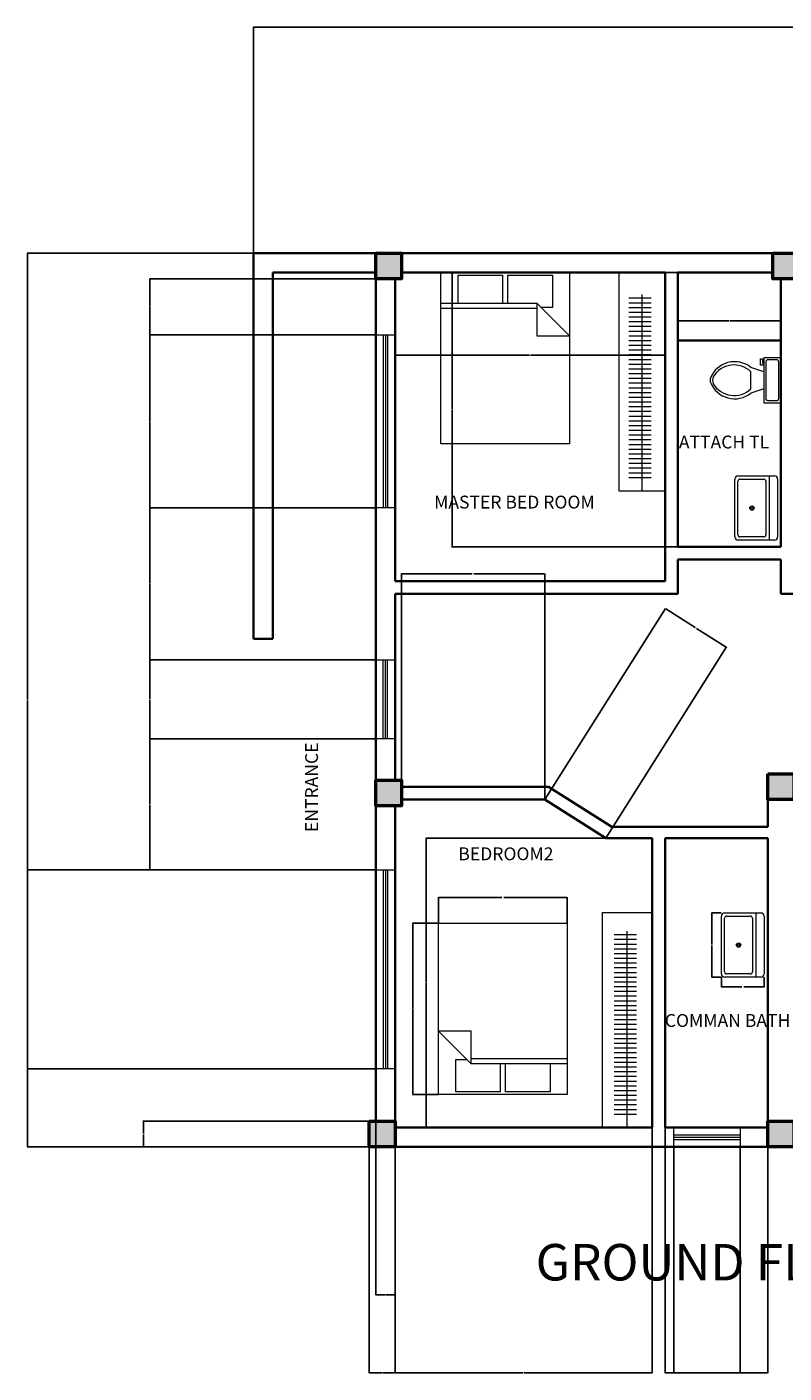
# Model space of a CAD drawing. Units: inches. Extents: x 369 to 4994, y 516 to 1297.
# Tile 1 of 9: x 369 to 722, y 516 to 1144. Entities that reach past the tile are written whole.
import ezdxf

# ---------------------------------------------------------------- set-up
doc = ezdxf.new("R2010")
doc.units = ezdxf.units.IN
doc.header["$MEASUREMENT"] = 0
for name, color, linetype, lineweight in [('A-ANNO-DIMS', 2, 'Continuous', 18), ('A-ANNO-TEXT', 7, 'Continuous', 35), ('A-AREA-IDEN', 7, 'Continuous', 18), ('A-COLS', 7, 'Continuous', 50), ('A-FLOR-CASE', 8, 'Continuous', 18), ('A-FLOR-CASE-PATT', 252, 'Continuous', 13), ('A-FLOR-FIXT', 9, 'Continuous', 18), ('A-FLOR-STRS', 3, 'Continuous', 25), ('A-FURN', 8, 'Continuous', 18), ('A-GLAZ', 4, 'Continuous', 18), ('A-WALL', 7, 'Continuous', 35)]:
    doc.layers.add(name, color=color, linetype=linetype, lineweight=lineweight)
doc.layers.add('A-COLS-PATT', color=18, linetype='Continuous', lineweight=13, true_color=0x000000)
doc.styles.get("Standard").update_dxf_attribs({"font": 'arial.ttf'})
doc.dimstyles.get("Standard").update_dxf_attribs({"dimtxt": 0.18, "dimasz": 0.18, "dimexe": 0.18, "dimexo": 0.0625, "dimgap": 0.09, "dimtad": 0, "dimtih": 1, "dimtoh": 1, "dimdec": 4, "dimzin": 0, "dimdsep": 46, "dimtxsty": 'Standard', "dimcen": 0.09, "dimadec": 0, "dimazin": 0, "dimtfac": 1, "dimtdec": 4, "dimtofl": 0, "dimtmove": 0, "dimatfit": 3, "dimfxl": 1, "dimtolj": 1, "dimtzin": 0, "dimarcsym": 0})

# ---------------------------------------------------------------- blocks, each defined once
blk = doc.blocks.new('Bed - Queen')
for p, q in [((0, -80.00003), (0, 0)), ((0, 0), (59.99999, 0)), ((59.99999, 0), (59.99999, -80.00003)), ((7.99999, -1.2), (28.79998, -1.2)), ((7.99999, -14.4), (7.99999, -1.2)), ((28.79998, -1.2), (28.79998, -14.4)), ((31.19999, -1.2), (51.99999, -1.2)), ((31.19999, -14.4), (31.19999, -1.2)), ((51.99999, -1.2), (51.99999, -16.4)), ((0, -14.4), (44.8, -14.4)), ((44.8, -16.8), (0, -16.8)), ((59.99999, -29.6), (44.8, -14.4)), ((44.8, -14.4), (44.8, -29.6)), ((51.99999, -16.4), (46.79936, -16.4)), ((44.8, -29.6), (59.99999, -29.6)), ((59.99999, -80.00003), (0, -80.00003))]:
    blk.add_line(p, q)
blk = doc.blocks.new('Toilet - top')
for p, q in [((9.5, -6), (9.5, -2)), ((-10, -8.5), (-8, -8.5)), ((-10, -9.5), (-10, -8.5)), ((-7, -9.5), (-10, -9.5)), ((-8, -8.5), (-8, -8)), ((-7, -8), (-7, -9.5)), ((-4, -8), (-6, -14)), ((4, -8), (6, -14)), ((4, -14), (-4, -14))]:
    blk.add_line(p, q)
blk.add_lwpolyline([(10.5, -8), (10.5, 0), (-10.5, 0), (-10.5, -8)], close=True)
for points in [[(-9.5, -2), (-9.5, -6)], [(8.5, -1), (-8.5, -1)], [(-8.5, -7), (8.5, -7)]]:
    blk.add_lwpolyline(points)
for centre, radius, start, end in [((-8.62, -1.88), 0.884, 81.8699, 188.1301), ((-8.62, -6.12), 0.884, 171.8699, 278.1301), ((8.62, -1.88), 0.884, 351.8699, 98.1301), ((8.62, -6.12), 0.884, 261.8699, 8.1301), ((3.52, -21.58), 12.17, 141.46911, 247.97143), ((4.2, -21.82), 11.33, 136.36773, 238.94682), ((-3.52, -21.58), 12.17, 292.02843, 38.53071), ((-4.2, -21.82), 11.33, 301.05301, 43.63209), ((0, -27.88), 4, 245.73182, 294.26817), ((0, -29), 4, 254.86053, 285.13947)]:
    blk.add_arc(centre, radius, start, end)
blk = doc.blocks.new('Sink-single - 30 in top')
blk.add_line((-15, -3.999996), (15, -3.999996))
for points in [[(-13.5, 0), (13.5, 0)], [(-15, -18.499996), (-15, -1.5)], [(-12.5, -5.499996), (12.5, -5.499996)], [(15, -1.5), (15, -18.499996)], [(-13.5, -17.499996), (-13.5, -6.499996)], [(13.5, -6.499996), (13.5, -17.499996)], [(12.5, -18.499996), (-12.5, -18.499996)], [(13.5, -19.999996), (-13.5, -19.999996)]]:
    blk.add_lwpolyline(points)
for radius in [1, 0.5]:
    blk.add_circle((0, -11.999996), radius)
for centre, radius, start, end in [((-13.5, -1.5), 1.5, 90, 180), ((-12.5, -6.499996), 1, 90, 180), ((12.5, -6.499996), 1, 0, 90), ((13.5, -1.5), 1.5, 0, 90), ((-13.5, -18.499996), 1.5, 180, 270), ((-12.5, -17.499996), 1, 180, 270), ((12.5, -17.499996), 1, 270, 0), ((13.5, -18.499996), 1.5, 270, 0)]:
    blk.add_arc(centre, radius, start, end)
blk = doc.blocks.new('BALCONY-EDGE')
for p, q in [((57, 180), (0, 180)), ((0, 180), (0, 0)), ((9, 171), (9, 0)), ((57, 171), (9, 171)), ((9, 0), (0, 0))]:
    blk.add_line(p, q)
blk = doc.blocks.new('*D19')
at = {"layer": 'A-ANNO-DIMS', "color": 0, "lineweight": -2, "transparency": 16777216}
for p, q in [((560.51, 726.18), (548.39, 726.18)), ((548.57, 726), (548.57, 686.37)), ((548.57, 646.36), (548.57, 685.99)), ((560.51, 646.18), (548.39, 646.18))]:
    blk.add_line(p, q, dxfattribs=at)
at = {"layer": 'A-ANNO-DIMS', "color": 0, "transparency": 16777216}
for points in [[(548.54, 726), (548.6, 726), (548.57, 726.18)], [(548.54, 646.36), (548.6, 646.36), (548.57, 646.18)]]:
    blk.add_solid(points, dxfattribs=at)
at = {"layer": 'Defpoints', "color": 0, "transparency": 16777216}
for p in [(560.57, 726.18), (548.57, 646.18), (560.57, 646.18)]:
    blk.add_point(p, dxfattribs=at)
at = {"layer": 'A-ANNO-DIMS', "color": 0, "transparency": 16777216, "insert": (548.57, 686.18), "char_height": 0.18, "attachment_point": 5}
blk.add_mtext('\\A1;QUEEN BED 80 TYP.', dxfattribs=at)
blk = doc.blocks.new('*D20')
at = {"layer": 'A-ANNO-DIMS', "color": 0, "lineweight": -2, "transparency": 16777216}
for p, q in [((560.57, 726.24), (560.57, 738.36)), ((560.75, 738.18), (590.05, 738.18)), ((620.39, 738.18), (591.1, 738.18)), ((620.57, 726.24), (620.57, 738.36))]:
    blk.add_line(p, q, dxfattribs=at)
at = {"layer": 'A-ANNO-DIMS', "color": 0, "transparency": 16777216}
for points in [[(560.75, 738.21), (560.75, 738.15), (560.57, 738.18)], [(620.39, 738.21), (620.39, 738.15), (620.57, 738.18)]]:
    blk.add_solid(points, dxfattribs=at)
at = {"layer": 'Defpoints', "color": 0, "transparency": 16777216}
for p in [(560.57, 738.18), (560.57, 726.18), (620.57, 726.18)]:
    blk.add_point(p, dxfattribs=at)
at = {"layer": 'A-ANNO-DIMS', "color": 0, "transparency": 16777216, "insert": (590.57, 738.18), "char_height": 0.18, "attachment_point": 5}
blk.add_mtext('\\A1;60 TYP.', dxfattribs=at)
blk = doc.blocks.new('*D27')
at = {"layer": 'A-ANNO-DIMS', "color": 0, "lineweight": -2, "transparency": 16777216}
for p, q in [((692.45, 730.94), (687.83, 730.94)), ((688.01, 730.76), (688.01, 716.12)), ((688.01, 701.12), (688.01, 715.75)), ((692.45, 700.94), (687.83, 700.94))]:
    blk.add_line(p, q, dxfattribs=at)
at = {"layer": 'A-ANNO-DIMS', "color": 0, "transparency": 16777216}
for points in [[(687.98, 730.76), (688.04, 730.76), (688.01, 730.94)], [(687.98, 701.12), (688.04, 701.12), (688.01, 700.94)]]:
    blk.add_solid(points, dxfattribs=at)
at = {"layer": 'Defpoints', "color": 0, "transparency": 16777216}
for p in [(692.51, 730.94), (688.01, 700.94), (692.51, 700.94)]:
    blk.add_point(p, dxfattribs=at)
at = {"layer": 'A-ANNO-DIMS', "color": 0, "transparency": 16777216, "insert": (688.01, 715.94), "char_height": 0.18, "attachment_point": 5}
blk.add_mtext('\\A1;SINK 30 TYP.', dxfattribs=at)
blk = doc.blocks.new('*D28')
at = {"layer": 'A-ANNO-DIMS', "color": 0, "lineweight": -2, "transparency": 16777216}
for p, q in [((692.51, 700.88), (692.51, 696.26)), ((712.51, 700.88), (712.51, 696.26)), ((692.69, 696.44), (701.98, 696.44)), ((712.33, 696.44), (703.04, 696.44))]:
    blk.add_line(p, q, dxfattribs=at)
at = {"layer": 'A-ANNO-DIMS', "color": 0, "transparency": 16777216}
for points in [[(692.69, 696.47), (692.69, 696.41), (692.51, 696.44)], [(712.33, 696.47), (712.33, 696.41), (712.51, 696.44)]]:
    blk.add_solid(points, dxfattribs=at)
at = {"layer": 'Defpoints', "color": 0, "transparency": 16777216}
for p in [(692.51, 700.94), (712.51, 700.94), (712.51, 696.44)]:
    blk.add_point(p, dxfattribs=at)
at = {"layer": 'A-ANNO-DIMS', "color": 0, "transparency": 16777216, "insert": (702.51, 696.44), "char_height": 0.18, "attachment_point": 5}
blk.add_mtext('\\A1;20 TYP.', dxfattribs=at)
blk = doc.blocks.new('*D39')
at = {"layer": 'A-ANNO-DIMS', "color": 0, "lineweight": -2, "transparency": 16777216}
for p, q in [((474.26, 1038.85), (474.26, 1144.37)), ((474.44, 1144.19), (760.47, 1144.19)), ((1047.08, 1144.19), (761.05, 1144.19)), ((1047.26, 1038.85), (1047.26, 1144.37))]:
    blk.add_line(p, q, dxfattribs=at)
at = {"layer": 'A-ANNO-DIMS', "color": 0, "transparency": 16777216}
for points in [[(474.44, 1144.22), (474.44, 1144.16), (474.26, 1144.19)], [(1047.08, 1144.22), (1047.08, 1144.16), (1047.26, 1144.19)]]:
    blk.add_solid(points, dxfattribs=at)
at = {"layer": 'Defpoints', "color": 0, "transparency": 16777216}
for p in [(1047.26, 1144.19), (474.26, 1038.79), (1047.26, 1038.79)]:
    blk.add_point(p, dxfattribs=at)
at = {"layer": 'A-ANNO-DIMS', "color": 0, "transparency": 16777216, "insert": (760.76, 1144.19), "char_height": 0.18, "attachment_point": 5}
blk.add_mtext('\\A1;573', dxfattribs=at)
blk = doc.blocks.new('*D40')
at = {"layer": 'A-ANNO-DIMS', "color": 0, "lineweight": -2, "transparency": 16777216}
for p, q in [((474.2, 1038.79), (368.68, 1038.79)), ((368.86, 1038.61), (368.86, 830.47)), ((368.86, 621.97), (368.86, 830.11)), ((528.2, 621.79), (368.68, 621.79))]:
    blk.add_line(p, q, dxfattribs=at)
at = {"layer": 'A-ANNO-DIMS', "color": 0, "transparency": 16777216}
for points in [[(368.83, 1038.61), (368.89, 1038.61), (368.86, 1038.79)], [(368.83, 621.97), (368.89, 621.97), (368.86, 621.79)]]:
    blk.add_solid(points, dxfattribs=at)
at = {"layer": 'Defpoints', "color": 0, "transparency": 16777216}
for p in [(368.86, 1038.79), (474.26, 1038.79), (528.26, 621.79)]:
    blk.add_point(p, dxfattribs=at)
at = {"layer": 'A-ANNO-DIMS', "color": 0, "transparency": 16777216, "insert": (368.86, 830.29), "char_height": 0.18, "attachment_point": 5}
blk.add_mtext('\\A1;417', dxfattribs=at)
blk = doc.blocks.new('*D41')
at = {"layer": 'A-ANNO-DIMS', "color": 0, "lineweight": -2, "transparency": 16777216}
for p, q in [((540.26, 885.85), (540.26, 991.37)), ((540.44, 991.19), (602.98, 991.19)), ((666.08, 991.19), (603.54, 991.19)), ((666.26, 885.85), (666.26, 991.37))]:
    blk.add_line(p, q, dxfattribs=at)
at = {"layer": 'A-ANNO-DIMS', "color": 0, "transparency": 16777216}
for points in [[(540.44, 991.22), (540.44, 991.16), (540.26, 991.19)], [(666.08, 991.22), (666.08, 991.16), (666.26, 991.19)]]:
    blk.add_solid(points, dxfattribs=at)
at = {"layer": 'Defpoints', "color": 0, "transparency": 16777216}
for p in [(666.26, 991.19), (540.26, 885.79), (666.26, 885.79)]:
    blk.add_point(p, dxfattribs=at)
at = {"layer": 'A-ANNO-DIMS', "color": 0, "transparency": 16777216, "insert": (603.26, 991.19), "char_height": 0.18, "attachment_point": 5}
blk.add_mtext('\\A1;126', dxfattribs=at)
blk = doc.blocks.new('*D42')
at = {"layer": 'A-ANNO-DIMS', "color": 0, "lineweight": -2, "transparency": 16777216}
for p, q in [((672.26, 901.88), (672.26, 1007.4)), ((672.44, 1007.22), (696.04, 1007.22)), ((720.08, 1007.22), (696.48, 1007.22)), ((720.26, 901.88), (720.26, 1007.4))]:
    blk.add_line(p, q, dxfattribs=at)
at = {"layer": 'A-ANNO-DIMS', "color": 0, "transparency": 16777216}
for points in [[(672.44, 1007.25), (672.44, 1007.19), (672.26, 1007.22)], [(720.08, 1007.25), (720.08, 1007.19), (720.26, 1007.22)]]:
    blk.add_solid(points, dxfattribs=at)
at = {"layer": 'Defpoints', "color": 0, "transparency": 16777216}
for p in [(720.26, 1007.22), (672.26, 901.82), (720.26, 901.82)]:
    blk.add_point(p, dxfattribs=at)
at = {"layer": 'A-ANNO-DIMS', "color": 0, "transparency": 16777216, "insert": (696.26, 1007.22), "char_height": 0.18, "attachment_point": 5}
blk.add_mtext('\\A1;48', dxfattribs=at)
blk = doc.blocks.new('*D48')
at = {"layer": 'A-ANNO-DIMS', "color": 0, "lineweight": -2, "transparency": 16777216}
for p, q in [((540.26, 630.73), (540.26, 516.21)), ((660.26, 630.73), (660.26, 516.21)), ((540.44, 516.39), (599.98, 516.39)), ((660.08, 516.39), (600.54, 516.39))]:
    blk.add_line(p, q, dxfattribs=at)
at = {"layer": 'A-ANNO-DIMS', "color": 0, "transparency": 16777216}
for points in [[(540.44, 516.42), (540.44, 516.36), (540.26, 516.39)], [(660.08, 516.42), (660.08, 516.36), (660.26, 516.39)]]:
    blk.add_solid(points, dxfattribs=at)
at = {"layer": 'Defpoints', "color": 0, "transparency": 16777216}
for p in [(540.26, 630.79), (660.26, 630.79), (660.26, 516.39)]:
    blk.add_point(p, dxfattribs=at)
at = {"layer": 'A-ANNO-DIMS', "color": 0, "transparency": 16777216, "insert": (600.26, 516.39), "char_height": 0.18, "attachment_point": 5}
blk.add_mtext('\\A1;120', dxfattribs=at)
blk = doc.blocks.new('*D49')
at = {"layer": 'A-ANNO-DIMS', "color": 0, "lineweight": -2, "transparency": 16777216}
for p, q in [((666.26, 630.73), (666.26, 516.21)), ((714.26, 630.73), (714.26, 516.21)), ((666.44, 516.39), (690.04, 516.39)), ((714.08, 516.39), (690.48, 516.39))]:
    blk.add_line(p, q, dxfattribs=at)
at = {"layer": 'A-ANNO-DIMS', "color": 0, "transparency": 16777216}
for points in [[(666.44, 516.42), (666.44, 516.36), (666.26, 516.39)], [(714.08, 516.42), (714.08, 516.36), (714.26, 516.39)]]:
    blk.add_solid(points, dxfattribs=at)
at = {"layer": 'Defpoints', "color": 0, "transparency": 16777216}
for p in [(666.26, 630.79), (714.26, 630.79), (714.26, 516.39)]:
    blk.add_point(p, dxfattribs=at)
at = {"layer": 'A-ANNO-DIMS', "color": 0, "transparency": 16777216, "insert": (690.26, 516.39), "char_height": 0.18, "attachment_point": 5}
blk.add_mtext('\\A1;48', dxfattribs=at)
blk = doc.blocks.new('*D53')
at = {"layer": 'A-ANNO-DIMS', "color": 0, "lineweight": -2, "transparency": 16777216}
for p, q in [((672.2, 1029.79), (566.68, 1029.79)), ((566.86, 1029.61), (566.86, 965.99)), ((566.86, 902), (566.86, 965.62)), ((672.2, 901.82), (566.68, 901.82))]:
    blk.add_line(p, q, dxfattribs=at)
at = {"layer": 'A-ANNO-DIMS', "color": 0, "transparency": 16777216}
for points in [[(566.83, 1029.61), (566.89, 1029.61), (566.86, 1029.79)], [(566.83, 902), (566.89, 902), (566.86, 901.82)]]:
    blk.add_solid(points, dxfattribs=at)
at = {"layer": 'Defpoints', "color": 0, "transparency": 16777216}
for p in [(566.86, 1029.79), (672.26, 1029.79), (672.26, 901.82)]:
    blk.add_point(p, dxfattribs=at)
at = {"layer": 'A-ANNO-DIMS', "color": 0, "transparency": 16777216, "insert": (566.86, 965.8), "char_height": 0.18, "attachment_point": 5}
blk.add_mtext('\\A1;127.97', dxfattribs=at)
blk = doc.blocks.new('*D56')
at = {"layer": 'A-ANNO-DIMS', "color": 0, "lineweight": -2, "transparency": 16777216}
for p, q in [((660.2, 765.79), (554.68, 765.79)), ((554.86, 765.61), (554.86, 698.47)), ((554.86, 630.97), (554.86, 698.11)), ((660.2, 630.79), (554.68, 630.79))]:
    blk.add_line(p, q, dxfattribs=at)
at = {"layer": 'A-ANNO-DIMS', "color": 0, "transparency": 16777216}
for points in [[(554.83, 765.61), (554.89, 765.61), (554.86, 765.79)], [(554.83, 630.97), (554.89, 630.97), (554.86, 630.79)]]:
    blk.add_solid(points, dxfattribs=at)
at = {"layer": 'Defpoints', "color": 0, "transparency": 16777216}
for p in [(554.86, 765.79), (660.26, 765.79), (660.26, 630.79)]:
    blk.add_point(p, dxfattribs=at)
at = {"layer": 'A-ANNO-DIMS', "color": 0, "transparency": 16777216, "insert": (554.86, 698.29), "char_height": 0.18, "attachment_point": 5}
blk.add_mtext('\\A1;135', dxfattribs=at)
blk = doc.blocks.new('*D57')
at = {"layer": 'A-ANNO-DIMS', "color": 0, "lineweight": -2, "transparency": 16777216}
for p, q in [((543.26, 783.85), (543.26, 889.37)), ((543.44, 889.19), (576.28, 889.19)), ((609.9, 889.19), (577.07, 889.19)), ((610.08, 783.85), (610.08, 889.37))]:
    blk.add_line(p, q, dxfattribs=at)
at = {"layer": 'A-ANNO-DIMS', "color": 0, "transparency": 16777216}
for points in [[(543.44, 889.22), (543.44, 889.16), (543.26, 889.19)], [(609.9, 889.22), (609.9, 889.16), (610.08, 889.19)]]:
    blk.add_solid(points, dxfattribs=at)
at = {"layer": 'Defpoints', "color": 0, "transparency": 16777216}
for p in [(610.08, 889.19), (543.26, 783.79), (610.08, 783.79)]:
    blk.add_point(p, dxfattribs=at)
at = {"layer": 'A-ANNO-DIMS', "color": 0, "transparency": 16777216, "insert": (576.67, 889.19), "char_height": 0.18, "attachment_point": 5}
blk.add_mtext('\\A1;66.83', dxfattribs=at)
blk = doc.blocks.new('*D58')
at = {"layer": 'A-ANNO-DIMS', "color": 0, "lineweight": -2, "transparency": 16777216}
for p, q in [((610.12, 783.84), (666.48, 873.04)), ((666.54, 872.8), (680.34, 864.07)), ((694.72, 854.99), (680.92, 863.71)), ((638.61, 765.84), (694.97, 855.04))]:
    blk.add_line(p, q, dxfattribs=at)
at = {"layer": 'A-ANNO-DIMS', "color": 0, "transparency": 16777216}
for points in [[(666.55, 872.82), (666.52, 872.77), (666.39, 872.89)], [(694.74, 855.01), (694.7, 854.96), (694.87, 854.89)]]:
    blk.add_solid(points, dxfattribs=at)
at = {"layer": 'Defpoints', "color": 0, "transparency": 16777216}
for p in [(694.87, 854.89), (610.08, 783.79), (638.57, 765.79)]:
    blk.add_point(p, dxfattribs=at)
at = {"layer": 'A-ANNO-DIMS', "color": 0, "transparency": 16777216, "insert": (680.63, 863.89), "char_height": 0.18, "attachment_point": 5}
blk.add_mtext('\\A1;33.7', dxfattribs=at)
blk = doc.blocks.new('*D59')
at = {"layer": 'A-ANNO-DIMS', "color": 0, "lineweight": -2, "transparency": 16777216}
for p, q in [((531.2, 1026.79), (425.68, 1026.79)), ((425.86, 1026.61), (425.86, 1013.94)), ((425.86, 1000.91), (425.86, 1013.58)), ((531.2, 1000.73), (425.68, 1000.73))]:
    blk.add_line(p, q, dxfattribs=at)
at = {"layer": 'A-ANNO-DIMS', "color": 0, "transparency": 16777216}
for points in [[(425.83, 1026.61), (425.89, 1026.61), (425.86, 1026.79)], [(425.83, 1000.91), (425.89, 1000.91), (425.86, 1000.73)]]:
    blk.add_solid(points, dxfattribs=at)
at = {"layer": 'Defpoints', "color": 0, "transparency": 16777216}
for p in [(425.86, 1026.79), (531.26, 1026.79), (531.26, 1000.73)]:
    blk.add_point(p, dxfattribs=at)
at = {"layer": 'A-ANNO-DIMS', "color": 0, "transparency": 16777216, "insert": (425.86, 1013.76), "char_height": 0.18, "attachment_point": 5}
blk.add_mtext('\\A1;26.06', dxfattribs=at)
blk = doc.blocks.new('*D60')
at = {"layer": 'A-ANNO-DIMS', "color": 0, "lineweight": -2, "transparency": 16777216}
for p, q in [((531.2, 1000.73), (425.68, 1000.73)), ((425.86, 1000.55), (425.86, 960.54)), ((425.86, 920.17), (425.86, 960.18)), ((531.2, 919.99), (425.68, 919.99))]:
    blk.add_line(p, q, dxfattribs=at)
at = {"layer": 'A-ANNO-DIMS', "color": 0, "transparency": 16777216}
for points in [[(425.83, 1000.55), (425.89, 1000.55), (425.86, 1000.73)], [(425.83, 920.17), (425.89, 920.17), (425.86, 919.99)]]:
    blk.add_solid(points, dxfattribs=at)
at = {"layer": 'Defpoints', "color": 0, "transparency": 16777216}
for p in [(425.86, 1000.73), (531.26, 1000.73), (531.26, 919.99)]:
    blk.add_point(p, dxfattribs=at)
at = {"layer": 'A-ANNO-DIMS', "color": 0, "transparency": 16777216, "insert": (425.86, 960.36), "char_height": 0.18, "attachment_point": 5}
blk.add_mtext('\\A1;80.74', dxfattribs=at)
blk = doc.blocks.new('*D61')
at = {"layer": 'A-ANNO-DIMS', "color": 0, "lineweight": -2, "transparency": 16777216}
for p, q in [((531.2, 919.99), (425.68, 919.99)), ((425.86, 919.81), (425.86, 884.72)), ((425.86, 849.26), (425.86, 884.35)), ((531.2, 849.08), (425.68, 849.08))]:
    blk.add_line(p, q, dxfattribs=at)
at = {"layer": 'A-ANNO-DIMS', "color": 0, "transparency": 16777216}
for points in [[(425.83, 919.81), (425.89, 919.81), (425.86, 919.99)], [(425.83, 849.26), (425.89, 849.26), (425.86, 849.08)]]:
    blk.add_solid(points, dxfattribs=at)
at = {"layer": 'Defpoints', "color": 0, "transparency": 16777216}
for p in [(425.86, 919.99), (531.26, 919.99), (531.26, 849.08)]:
    blk.add_point(p, dxfattribs=at)
at = {"layer": 'A-ANNO-DIMS', "color": 0, "transparency": 16777216, "insert": (425.86, 884.54), "char_height": 0.18, "attachment_point": 5}
blk.add_mtext('\\A1;70.91', dxfattribs=at)
blk = doc.blocks.new('*D62')
at = {"layer": 'A-ANNO-DIMS', "color": 0, "lineweight": -2, "transparency": 16777216}
for p, q in [((531.2, 849.08), (425.68, 849.08)), ((425.86, 848.9), (425.86, 830.78)), ((425.86, 812.3), (425.86, 830.42)), ((531.2, 812.12), (425.68, 812.12))]:
    blk.add_line(p, q, dxfattribs=at)
at = {"layer": 'A-ANNO-DIMS', "color": 0, "transparency": 16777216}
for points in [[(425.83, 848.9), (425.89, 848.9), (425.86, 849.08)], [(425.83, 812.3), (425.89, 812.3), (425.86, 812.12)]]:
    blk.add_solid(points, dxfattribs=at)
at = {"layer": 'Defpoints', "color": 0, "transparency": 16777216}
for p in [(425.86, 849.08), (531.26, 849.08), (531.26, 812.12)]:
    blk.add_point(p, dxfattribs=at)
at = {"layer": 'A-ANNO-DIMS', "color": 0, "transparency": 16777216, "insert": (425.86, 830.6), "char_height": 0.18, "attachment_point": 5}
blk.add_mtext('\\A1;36.96', dxfattribs=at)
blk = doc.blocks.new('*D63')
at = {"layer": 'A-ANNO-DIMS', "color": 0, "lineweight": -2, "transparency": 16777216}
for p, q in [((531.2, 812.12), (425.68, 812.12)), ((425.86, 811.94), (425.86, 781.79)), ((425.86, 751.28), (425.86, 781.43)), ((531.2, 751.1), (425.68, 751.1))]:
    blk.add_line(p, q, dxfattribs=at)
at = {"layer": 'A-ANNO-DIMS', "color": 0, "transparency": 16777216}
for points in [[(425.83, 811.94), (425.89, 811.94), (425.86, 812.12)], [(425.83, 751.28), (425.89, 751.28), (425.86, 751.1)]]:
    blk.add_solid(points, dxfattribs=at)
at = {"layer": 'Defpoints', "color": 0, "transparency": 16777216}
for p in [(425.86, 812.12), (531.26, 812.12), (531.26, 751.1)]:
    blk.add_point(p, dxfattribs=at)
at = {"layer": 'A-ANNO-DIMS', "color": 0, "transparency": 16777216, "insert": (425.86, 781.61), "char_height": 0.18, "attachment_point": 5}
blk.add_mtext('\\A1;61.02', dxfattribs=at)
blk = doc.blocks.new('*D64')
at = {"layer": 'A-ANNO-DIMS', "color": 0, "lineweight": -2, "transparency": 16777216}
for p, q in [((531.2, 751.1), (368.68, 751.1)), ((368.86, 750.92), (368.86, 704.82)), ((368.86, 658.37), (368.86, 704.46)), ((531.2, 658.19), (368.68, 658.19))]:
    blk.add_line(p, q, dxfattribs=at)
at = {"layer": 'A-ANNO-DIMS', "color": 0, "transparency": 16777216}
for points in [[(368.83, 750.92), (368.89, 750.92), (368.86, 751.1)], [(368.83, 658.37), (368.89, 658.37), (368.86, 658.19)]]:
    blk.add_solid(points, dxfattribs=at)
at = {"layer": 'Defpoints', "color": 0, "transparency": 16777216}
for p in [(368.86, 751.1), (531.26, 751.1), (531.26, 658.19)]:
    blk.add_point(p, dxfattribs=at)
at = {"layer": 'A-ANNO-DIMS', "color": 0, "transparency": 16777216, "insert": (368.86, 704.64), "char_height": 0.18, "attachment_point": 5}
blk.add_mtext('\\A1;92.91', dxfattribs=at)
blk = doc.blocks.new('*D68')
at = {"layer": 'A-ANNO-DIMS', "color": 0, "lineweight": -2, "transparency": 16777216}
for p, q in [((670.31, 621.73), (670.31, 516.21)), ((701.35, 621.73), (701.35, 516.21)), ((670.49, 516.39), (685.44, 516.39)), ((701.17, 516.39), (686.22, 516.39))]:
    blk.add_line(p, q, dxfattribs=at)
at = {"layer": 'A-ANNO-DIMS', "color": 0, "transparency": 16777216}
for points in [[(670.49, 516.42), (670.49, 516.36), (670.31, 516.39)], [(701.17, 516.42), (701.17, 516.36), (701.35, 516.39)]]:
    blk.add_solid(points, dxfattribs=at)
at = {"layer": 'Defpoints', "color": 0, "transparency": 16777216}
for p in [(670.31, 621.79), (701.35, 621.79), (701.35, 516.39)]:
    blk.add_point(p, dxfattribs=at)
at = {"layer": 'A-ANNO-DIMS', "color": 0, "transparency": 16777216, "insert": (685.83, 516.39), "char_height": 0.18, "attachment_point": 5}
blk.add_mtext('\\A1;31.04', dxfattribs=at)
blk = doc.blocks.new('*D69')
at = {"layer": 'A-ANNO-DIMS', "color": 0, "lineweight": -2, "transparency": 16777216}
for p, q in [((528.26, 621.73), (528.26, 516.21)), ((540.26, 621.73), (540.26, 516.21)), ((528.44, 516.39), (534.05, 516.39)), ((540.08, 516.39), (534.47, 516.39))]:
    blk.add_line(p, q, dxfattribs=at)
at = {"layer": 'A-ANNO-DIMS', "color": 0, "transparency": 16777216}
for points in [[(528.44, 516.42), (528.44, 516.36), (528.26, 516.39)], [(540.08, 516.42), (540.08, 516.36), (540.26, 516.39)]]:
    blk.add_solid(points, dxfattribs=at)
at = {"layer": 'Defpoints', "color": 0, "transparency": 16777216}
for p in [(528.26, 621.79), (540.26, 621.79), (528.26, 516.39)]:
    blk.add_point(p, dxfattribs=at)
at = {"layer": 'A-ANNO-DIMS', "color": 0, "transparency": 16777216, "insert": (534.26, 516.39), "char_height": 0.18, "attachment_point": 5}
blk.add_mtext('\\A1;12', dxfattribs=at)
blk = doc.blocks.new('*D70')
at = {"layer": 'A-ANNO-DIMS', "color": 0, "lineweight": -2, "transparency": 16777216}
for p, q in [((528.2, 633.79), (422.68, 633.79)), ((422.86, 633.61), (422.86, 627.97)), ((422.86, 621.97), (422.86, 627.61)), ((528.2, 621.79), (422.68, 621.79))]:
    blk.add_line(p, q, dxfattribs=at)
at = {"layer": 'A-ANNO-DIMS', "color": 0, "transparency": 16777216}
for points in [[(422.83, 633.61), (422.89, 633.61), (422.86, 633.79)], [(422.83, 621.97), (422.89, 621.97), (422.86, 621.79)]]:
    blk.add_solid(points, dxfattribs=at)
at = {"layer": 'Defpoints', "color": 0, "transparency": 16777216}
for p in [(422.86, 633.79), (528.26, 633.79), (528.26, 621.79)]:
    blk.add_point(p, dxfattribs=at)
at = {"layer": 'A-ANNO-DIMS', "color": 0, "transparency": 16777216, "insert": (422.86, 627.79), "char_height": 0.18, "attachment_point": 5}
blk.add_mtext('\\A1;12', dxfattribs=at)
blk = doc.blocks.new('*D71')
at = {"layer": 'A-ANNO-DIMS', "color": 0, "lineweight": -2, "transparency": 16777216}
for p, q in [((531.26, 658.12), (531.26, 552.61)), ((540.26, 658.12), (540.26, 552.61)), ((531.44, 552.79), (535.61, 552.79)), ((540.08, 552.79), (535.91, 552.79))]:
    blk.add_line(p, q, dxfattribs=at)
at = {"layer": 'A-ANNO-DIMS', "color": 0, "transparency": 16777216}
for points in [[(531.44, 552.82), (531.44, 552.76), (531.26, 552.79)], [(540.08, 552.82), (540.08, 552.76), (540.26, 552.79)]]:
    blk.add_solid(points, dxfattribs=at)
at = {"layer": 'Defpoints', "color": 0, "transparency": 16777216}
for p in [(531.26, 658.19), (540.26, 658.19), (531.26, 552.79)]:
    blk.add_point(p, dxfattribs=at)
at = {"layer": 'A-ANNO-DIMS', "color": 0, "transparency": 16777216, "insert": (535.76, 552.79), "char_height": 0.18, "attachment_point": 5}
blk.add_mtext('\\A1;9', dxfattribs=at)
blk = doc.blocks.new('*D75')
at = {"layer": 'A-ANNO-DIMS', "color": 0, "lineweight": -2, "transparency": 16777216}
for p, q in [((1208.31, 1038.79), (368.68, 1038.79)), ((368.86, 1038.61), (368.86, 830.47)), ((368.86, 621.97), (368.86, 830.11)), ((1262.31, 621.79), (368.68, 621.79))]:
    blk.add_line(p, q, dxfattribs=at)
at = {"layer": 'A-ANNO-DIMS', "color": 0, "transparency": 16777216}
for points in [[(368.83, 1038.61), (368.89, 1038.61), (368.86, 1038.79)], [(368.83, 621.97), (368.89, 621.97), (368.86, 621.79)]]:
    blk.add_solid(points, dxfattribs=at)
at = {"layer": 'Defpoints', "color": 0, "transparency": 16777216}
for p in [(368.86, 1038.79), (1208.37, 1038.79), (1262.37, 621.79)]:
    blk.add_point(p, dxfattribs=at)
at = {"layer": 'A-ANNO-DIMS', "color": 0, "transparency": 16777216, "insert": (368.86, 830.29), "char_height": 0.18, "attachment_point": 5}
blk.add_mtext('\\A1;417', dxfattribs=at)
blk = doc.blocks.new('*D98')
at = {"layer": 'A-ANNO-DIMS', "color": 0, "lineweight": -2, "transparency": 16777216}
for p, q in [((1992.86, 1038.79), (368.68, 1038.79)), ((368.86, 1038.61), (368.86, 830.47)), ((368.86, 621.97), (368.86, 830.11)), ((2046.86, 621.79), (368.68, 621.79))]:
    blk.add_line(p, q, dxfattribs=at)
at = {"layer": 'A-ANNO-DIMS', "color": 0, "transparency": 16777216}
for points in [[(368.83, 1038.61), (368.89, 1038.61), (368.86, 1038.79)], [(368.83, 621.97), (368.89, 621.97), (368.86, 621.79)]]:
    blk.add_solid(points, dxfattribs=at)
at = {"layer": 'Defpoints', "color": 0, "transparency": 16777216}
for p in [(368.86, 1038.79), (1992.93, 1038.79), (2046.93, 621.79)]:
    blk.add_point(p, dxfattribs=at)
at = {"layer": 'A-ANNO-DIMS', "color": 0, "transparency": 16777216, "insert": (368.86, 830.29), "char_height": 0.18, "attachment_point": 5}
blk.add_mtext('\\A1;417', dxfattribs=at)

msp = doc.modelspace()

# ---------------------------------------------------------------- hatches: boundary and pattern name
at = {"layer": 'A-COLS-PATT'}
h = msp.add_hatch(color=256, dxfattribs=at)
h.dxf.hatch_style = 1
h.paths.add_polyline_path([(540.2581, 633.7894), (528.2581, 633.7894), (528.2581, 621.7894), (540.2581, 621.7894)])
h.paths.add_polyline_path([(726.2581, 633.7894), (714.2581, 633.7894), (714.2581, 621.7894), (726.2581, 621.7894)])
h.paths.add_polyline_path([(918.2581, 633.7894), (906.2581, 633.7894), (906.2581, 621.7894), (918.2581, 621.7894)])
h.paths.add_polyline_path([(1047.2581, 633.7894), (1035.2581, 633.7894), (1035.2581, 621.7894), (1047.2581, 621.7894)])
h.paths.add_polyline_path([(1047.2581, 798.6977), (1035.2581, 798.6977), (1035.2581, 786.6977), (1047.2581, 786.6977)])
h.paths.add_polyline_path([(918.2581, 795.7894), (906.2581, 795.7894), (906.2581, 783.7894), (918.2581, 783.7894)])
h.paths.add_polyline_path([(726.2581, 795.7894), (714.2581, 795.7894), (714.2581, 783.7894), (726.2581, 783.7894)])
h.paths.add_polyline_path([(1047.2581, 1038.7894), (1035.2581, 1038.7894), (1035.2581, 1026.7894), (1047.2581, 1026.7894)])
h.paths.add_polyline_path([(855.044, 1038.7894), (843.044, 1038.7894), (843.044, 1026.7894), (855.044, 1026.7894)])
h.paths.add_polyline_path([(728.5536, 1038.7894), (716.5536, 1038.7894), (716.5536, 1026.7894), (728.5536, 1026.7894)])
h.paths.add_polyline_path([(543.2581, 1038.7894), (531.2581, 1038.7894), (531.2581, 1026.7894), (543.2581, 1026.7894)])
h.paths.add_polyline_path([(543.2581, 792.9013), (531.2581, 792.9013), (531.2581, 780.9013), (543.2581, 780.9013), (543.2581, 783.7894)])
h.paths.add_polyline_path([(1274.3738, 633.7894), (1262.3738, 633.7894), (1262.3738, 621.7894), (1274.3738, 621.7894)])
h.paths.add_polyline_path([(1460.3738, 633.7894), (1448.3738, 633.7894), (1448.3738, 621.7894), (1460.3738, 621.7894)])
h.paths.add_polyline_path([(1652.3738, 633.7894), (1640.3738, 633.7894), (1640.3738, 621.7894), (1652.3738, 621.7894)])
h.paths.add_polyline_path([(1781.3738, 633.7894), (1769.3738, 633.7894), (1769.3738, 621.7894), (1781.3738, 621.7894)])
h.paths.add_polyline_path([(1781.3738, 1038.7894), (1769.3738, 1038.7894), (1769.3738, 1026.7894), (1781.3738, 1026.7894)])
h.paths.add_polyline_path([(1625.484, 1038.7894), (1613.484, 1038.7894), (1613.484, 1026.7894), (1615.6962, 1026.7894), (1625.484, 1026.7894)])
h.paths.add_polyline_path([(1462.6692, 1038.7894), (1450.6692, 1038.7894), (1450.6692, 1026.7894), (1462.6692, 1026.7894)])
h.paths.add_polyline_path([(1277.3738, 1038.7894), (1265.3738, 1038.7894), (1265.3738, 1026.7894), (1277.3738, 1026.7894)])
h.paths.add_polyline_path([(1460.3738, 807.7894), (1448.3738, 807.7894), (1448.3738, 795.7894), (1460.3738, 795.7894)])
h.paths.add_polyline_path([(1652.3738, 807.7894), (1640.3738, 807.7894), (1640.3738, 795.7894), (1652.3738, 795.7894)])
h.paths.add_polyline_path([(2244.9265, 633.7894), (2232.9265, 633.7894), (2232.9265, 621.7894), (2244.9265, 621.7894)])
h.paths.add_polyline_path([(2058.9265, 633.7894), (2046.9265, 633.7894), (2046.9265, 621.7894), (2058.9265, 621.7894)])
h.paths.add_polyline_path([(2436.9265, 633.7894), (2424.9265, 633.7894), (2424.9265, 621.7894), (2436.9265, 621.7894)])
h.paths.add_polyline_path([(2565.9265, 633.7894), (2553.9265, 633.7894), (2553.9265, 621.7894), (2565.9265, 621.7894)])
h.paths.add_polyline_path([(2565.9265, 798.6977), (2553.9265, 798.6977), (2553.9265, 786.6977), (2565.9265, 786.6977)])
h.paths.add_polyline_path([(2565.9265, 1038.7894), (2553.9265, 1038.7894), (2553.9265, 1026.7894), (2565.9265, 1026.7894)])
h.paths.add_polyline_path([(2436.9265, 1038.7894), (2424.9265, 1038.7894), (2424.9265, 1026.7894), (2436.9265, 1026.7894)])
h.paths.add_polyline_path([(2247.222, 1038.7894), (2235.222, 1038.7894), (2235.222, 1026.7894), (2247.222, 1026.7894)])
h.paths.add_polyline_path([(2061.9265, 1038.7894), (2049.9265, 1038.7894), (2049.9265, 1026.7894), (2061.9265, 1026.7894)])
at = {"layer": 'A-FLOR-CASE-PATT'}
h = msp.add_hatch(dxfattribs=at)
h.set_pattern_fill('ANSI31', color=256, scale=17.6257, angle=-45, style=0)
h.paths.add_polyline_path([(649.373, 932.9574), (659.741, 932.9574), (659.741, 1018.8186), (649.373, 1018.8186)])
h = msp.add_hatch(dxfattribs=at)
h.set_pattern_fill('ANSI31', color=256, scale=17.6351, angle=-45, style=0)
h.paths.add_polyline_path([(642.516, 635.8858), (652.884, 635.8858), (652.884, 721.7472), (642.516, 721.7472)])

# ---------------------------------------------------------------- linework, layer by layer
at = {"layer": 'A-COLS'}
for points in [[(531.2581, 1038.7894), (543.2581, 1038.7894), (543.2581, 1026.7894), (531.2581, 1026.7894)], [(716.5536, 1038.7894), (728.5536, 1038.7894), (728.5536, 1026.7894), (716.5536, 1026.7894)], [(714.2581, 795.7894), (726.2581, 795.7894), (726.2581, 783.7894), (714.2581, 783.7894)], [(528.2581, 633.7894), (540.2581, 633.7894), (540.2581, 621.7894), (528.2581, 621.7894)]]:
    msp.add_lwpolyline(points, close=True, dxfattribs=at)
for points in [[(543.2581, 783.7894), (543.2581, 780.9013), (531.2581, 780.9013), (531.2581, 792.9013), (543.2581, 792.9013), (543.2581, 783.7894)], [(726.2581, 621.7894), (714.2581, 621.7894), (714.2581, 633.7894), (726.2581, 633.7894), (726.2581, 621.7894)]]:
    msp.add_lwpolyline(points, dxfattribs=at)
at = {"layer": 'A-FLOR-CASE'}
for p, q in [((655.4928, 927.8608), (655.4928, 1019.5638)), ((648.6358, 630.7894), (648.6358, 722.4923))]:
    msp.add_line(p, q, dxfattribs=at)
for points in [[(666.2581, 1029.7894), (644.7274, 1029.7894), (644.7274, 927.8608), (666.2581, 927.8608)], [(660.2581, 630.7894), (637.0134, 630.7894), (637.0134, 731.202), (660.2581, 731.202)]]:
    msp.add_lwpolyline(points, close=True, dxfattribs=at)
at = {"layer": 'A-FLOR-STRS'}
msp.add_line((726.2581, 795.7894), (714.2581, 795.7894), dxfattribs=at)
at = {"layer": 'A-GLAZ'}
for p, q in [((534.6821, 1000.7306), (534.6821, 919.9908)), ((535.7581, 1000.7306), (535.7581, 919.9908)), ((536.8342, 1000.7306), (536.8342, 919.9908)), ((534.6821, 812.119), (534.6821, 849.0806)), ((535.7581, 812.119), (535.7581, 849.0806)), ((536.8342, 812.119), (536.8342, 849.0806)), ((534.6821, 751.0967), (534.6821, 658.186)), ((535.7581, 751.0967), (535.7581, 658.186)), ((536.8342, 751.0967), (536.8342, 658.186)), ((670.311, 627.3655), (701.35, 627.3655)), ((670.311, 626.2894), (701.35, 626.2894)), ((670.311, 625.2133), (701.35, 625.2133))]:
    msp.add_line(p, q, dxfattribs=at)
for points in [[(540.2581, 919.9908), (531.2581, 919.9908), (531.2581, 1000.7306), (540.2581, 1000.7306)], [(540.2581, 812.119), (531.2581, 812.119), (531.2581, 849.0806), (540.2581, 849.0806)], [(540.2581, 658.186), (531.2581, 658.186), (531.2581, 751.0967), (540.2581, 751.0967)], [(670.311, 630.7894), (701.35, 630.7894), (701.35, 621.7894), (670.311, 621.7894)]]:
    msp.add_lwpolyline(points, close=True, dxfattribs=at)
at = {"layer": 'A-WALL'}
for p, q in [((1038.2581, 1038.7894), (531.2581, 1038.7894)), ((531.2581, 1029.7894), (531.2581, 633.7894)), ((540.2581, 885.7894), (540.2581, 1026.7894)), ((666.2581, 1029.7894), (543.2581, 1029.7894)), ((666.2581, 1029.7894), (666.2581, 885.7894)), ((716.5536, 1029.7894), (672.2581, 1029.7894)), ((672.2581, 1029.7894), (672.2581, 901.8196)), ((720.2581, 1026.7894), (720.2581, 901.8196)), ((672.2581, 997.9927), (720.2581, 997.9927)), ((672.2581, 901.8196), (720.2581, 901.8196)), ((672.2581, 895.8196), (720.2581, 895.8196)), ((672.2581, 895.8196), (672.2581, 879.7894)), ((720.2581, 895.8196), (720.2581, 879.7894)), ((540.2581, 885.7894), (642.4388, 885.7894)), ((666.2581, 885.7894), (642.4388, 885.7894)), ((540.2581, 879.7894), (642.4388, 879.7894)), ((540.2581, 792.9013), (540.2581, 879.7894)), ((642.4388, 879.7894), (666.2581, 879.7894)), ((666.2581, 879.7894), (672.2581, 879.7894)), ((720.2581, 879.7894), (852.2581, 879.7894)), ((540.2581, 792.9013), (540.2581, 849.7894)), ((714.2581, 771.1277), (714.2581, 795.7894)), ((543.2581, 789.7894), (611.8215, 789.7894)), ((611.8215, 789.7894), (641.3562, 771.1277)), ((540.2581, 780.9013), (540.2581, 633.7894)), ((543.2581, 783.7894), (610.0848, 783.7894)), ((610.0848, 783.7894), (638.5723, 765.7894)), ((641.3562, 771.1277), (660.2581, 771.1277)), ((660.2581, 771.1277), (714.2581, 771.1277)), ((660.2581, 765.7894), (638.5723, 765.7894)), ((660.2581, 630.7894), (660.2581, 765.7894)), ((666.2581, 630.7894), (666.2581, 765.7894)), ((714.2581, 765.7894), (666.2581, 765.7894)), ((714.2581, 621.7894), (714.2581, 765.7894)), ((540.2581, 630.7894), (660.2581, 630.7894)), ((666.2581, 630.7894), (714.2581, 630.7894)), ((540.2581, 621.7894), (660.2581, 621.7894)), ((660.2581, 621.7894), (714.2581, 621.7894))]:
    msp.add_line(p, q, dxfattribs=at)

# ---------------------------------------------------------------- block references
at = {"layer": 'A-FLOR-FIXT', "rotation": 269.9999999999999}
for name, p in [('Toilet - top', (720.2581, 979.4994)), ('Sink-single - 30 in top', (718.7665, 919.861)), ('Sink-single - 30 in top', (712.5109, 715.938))]:
    msp.add_blockref(name, p, dxfattribs=at)
at = {"layer": 'A-FURN'}
msp.add_blockref('Bed - Queen', (561.6742, 1029.7894), dxfattribs=at)
at = {"layer": 'A-FURN', "rotation": 180}
msp.add_blockref('Bed - Queen', (620.5739, 646.1814), dxfattribs=at)
at = {"layer": 'A-WALL'}
msp.add_blockref('BALCONY-EDGE', (474.258, 858.789), dxfattribs=at)

# ---------------------------------------------------------------- texts
at = {"layer": 'A-ANNO-TEXT'}
msp.add_text('GROUND FLOOR ', height=17.017766, dxfattribs=at).set_placement((605.8748, 559.4225))
at = {"layer": 'A-AREA-IDEN'}
for s, p in [('ATTACH TL ', (672.6804, 947.6698)), ('MASTER BED ROOM', (558.5004, 919.642)), ('BEDROOM2  ', (569.8101, 755.5144)), ('COMMAN BATH ', (666.1342, 677.737))]:
    msp.add_text(s, height=6, dxfattribs=at).set_placement(p)
msp.add_text('ENTRANCE', height=6, rotation=90, dxfattribs=at).set_placement((504.3454, 768.6802))

# ---------------------------------------------------------------- dimensions: what is measured, and where the dimension line sits
at = {"layer": 'A-ANNO-DIMS'}
for base, p1, p2, override, picture, middle in [((1047.2581, 1144.1894), (474.2581, 1038.7894), (1047.2581, 1038.7894), {"dimdec": 0, "dimlfac": 1, "dimrnd": 0, "dimzin": 0, "dimdsep": 46, "dimlunit": 2}, '*D39', (760.7581, 1144.1894)), ((720.2581, 1007.2196), (672.2581, 901.8196), (720.2581, 901.8196), {"dimdec": 0, "dimlfac": 1, "dimrnd": 0, "dimzin": 0, "dimdsep": 46, "dimlunit": 2}, '*D42', (696.2581, 1007.2196)), ((666.2581, 991.1894), (540.2581, 885.7894), (666.2581, 885.7894), {"dimdec": 0, "dimlfac": 1, "dimrnd": 0, "dimzin": 0, "dimdsep": 46, "dimlunit": 2}, '*D41', (603.2581, 991.1894)), ((610.0848, 889.1894), (543.2581, 783.7894), (610.0848, 783.7894), {"dimdec": 2, "dimlfac": 1, "dimrnd": 0, "dimzin": 0, "dimdsep": 46, "dimlunit": 2}, '*D57', (576.6715, 889.1894)), ((660.2581, 516.3894), (540.2581, 630.7894), (660.2581, 630.7894), {"dimdec": 0, "dimlfac": 1, "dimrnd": 0, "dimzin": 0, "dimdsep": 46, "dimlunit": 2}, '*D48', (600.2581, 516.3894)), ((714.2581, 516.3894), (666.2581, 630.7894), (714.2581, 630.7894), {"dimdec": 0, "dimlfac": 1, "dimrnd": 0, "dimzin": 0, "dimdsep": 46, "dimlunit": 2}, '*D49', (690.2581, 516.3894)), ((701.35, 516.3894), (670.311, 621.7894), (701.35, 621.7894), {"dimdec": 2, "dimlfac": 1, "dimrnd": 0, "dimzin": 0, "dimdsep": 46, "dimlunit": 2}, '*D68', (685.8305, 516.3894))]:
    dim = msp.add_linear_dim(base=base, p1=p1, p2=p2, dimstyle='Standard', override=override, dxfattribs=at)
    dim.commit()
    dim.dimension.update_dxf_attribs({"geometry": picture, "text_midpoint": middle})
for base, p1, p2, angle, override, picture, middle in [((368.8581, 1038.7894), (528.2581, 621.7894), (474.2581, 1038.7894), 90, {"dimdec": 0, "dimlfac": 1, "dimrnd": 0, "dimzin": 0, "dimdsep": 46, "dimlunit": 2}, '*D40', (368.8581, 830.2894)), ((368.8581, 1038.7894), (1262.3738, 621.7894), (1208.3738, 1038.7894), 90, {"dimdec": 0, "dimlfac": 1, "dimrnd": 0, "dimzin": 0, "dimdsep": 46, "dimlunit": 2}, '*D75', (368.8581, 830.2894)), ((368.8581, 1038.7894), (2046.9265, 621.7894), (1992.9265, 1038.7894), 90, {"dimdec": 0, "dimlfac": 1, "dimrnd": 0, "dimzin": 0, "dimdsep": 46, "dimlunit": 2}, '*D98', (368.8581, 830.2894)), ((425.8581, 1026.7894), (531.2581, 1000.7306), (531.2581, 1026.7894), 90, {"dimdec": 2, "dimlfac": 1, "dimrnd": 0, "dimzin": 0, "dimdsep": 46, "dimlunit": 2}, '*D59', (425.8581, 1013.76)), ((566.8581, 1029.7894), (672.2581, 901.8196), (672.2581, 1029.7894), 90, {"dimdec": 2, "dimlfac": 1, "dimrnd": 0, "dimzin": 0, "dimdsep": 46, "dimlunit": 2}, '*D53', (566.8581, 965.8045)), ((425.8581, 1000.7306), (531.2581, 919.9908), (531.2581, 1000.7306), 90, {"dimdec": 2, "dimlfac": 1, "dimrnd": 0, "dimzin": 0, "dimdsep": 46, "dimlunit": 2}, '*D60', (425.8581, 960.3607)), ((425.8581, 919.9908), (531.2581, 849.0806), (531.2581, 919.9908), 90, {"dimdec": 2, "dimlfac": 1, "dimrnd": 0, "dimzin": 0, "dimdsep": 46, "dimlunit": 2}, '*D61', (425.8581, 884.5357)), ((694.8728, 854.8927), (610.0848, 783.7894), (638.5723, 765.7894), 327.7129888, {"dimdec": 1, "dimlfac": 1, "dimrnd": 0, "dimzin": 0, "dimdsep": 46, "dimlunit": 2}, '*D58', (680.6291, 863.8927)), ((425.8581, 849.0806), (531.2581, 812.119), (531.2581, 849.0806), 90, {"dimdec": 2, "dimlfac": 1, "dimrnd": 0, "dimzin": 0, "dimdsep": 46, "dimlunit": 2}, '*D62', (425.8581, 830.5998)), ((425.8581, 812.119), (531.2581, 751.0967), (531.2581, 812.119), 90, {"dimdec": 2, "dimlfac": 1, "dimrnd": 0, "dimzin": 0, "dimdsep": 46, "dimlunit": 2}, '*D63', (425.8581, 781.6079)), ((554.8581, 765.7894), (660.2581, 630.7894), (660.2581, 765.7894), 90, {"dimdec": 0, "dimlfac": 1, "dimrnd": 0, "dimzin": 0, "dimdsep": 46, "dimlunit": 2}, '*D56', (554.8581, 698.2894)), ((368.8581, 751.0967), (531.2581, 658.186), (531.2581, 751.0967), 90, {"dimdec": 2, "dimlfac": 1, "dimrnd": 0, "dimzin": 0, "dimdsep": 46, "dimlunit": 2}, '*D64', (368.8581, 704.6414)), ((531.2581, 552.786), (540.2581, 658.186), (531.2581, 658.186), 180, {"dimdec": 0, "dimlfac": 1, "dimrnd": 0, "dimzin": 0, "dimdsep": 46, "dimlunit": 2}, '*D71', (535.7581, 552.786)), ((422.8581, 633.7894), (528.2581, 621.7894), (528.2581, 633.7894), 90, {"dimdec": 0, "dimlfac": 1, "dimrnd": 0, "dimzin": 0, "dimdsep": 46, "dimlunit": 2}, '*D70', (422.8581, 627.7894)), ((528.2581, 516.3894), (540.2581, 621.7894), (528.2581, 621.7894), 180, {"dimdec": 0, "dimlfac": 1, "dimrnd": 0, "dimzin": 0, "dimdsep": 46, "dimlunit": 2}, '*D69', (534.2581, 516.3894))]:
    dim = msp.add_linear_dim(base=base, p1=p1, p2=p2, angle=angle, dimstyle='Standard', override=override, dxfattribs=at)
    dim.commit()
    dim.dimension.update_dxf_attribs({"geometry": picture, "text_midpoint": middle})
for base, p1, p2, angle, text, picture, middle in [((560.5739, 738.1815), (620.5739, 726.1814), (560.5739, 726.1814), 180, '<> TYP.', '*D20', (590.5739, 738.1815)), ((688.0109, 700.938), (692.5109, 730.938), (692.5109, 700.938), 270, 'SINK <> TYP.', '*D27', (688.0109, 715.938)), ((548.5739, 646.1814), (560.5739, 726.1814), (560.5739, 646.1814), 270, 'QUEEN BED <> TYP.', '*D19', (548.5739, 686.1814))]:
    dim = msp.add_linear_dim(base=base, p1=p1, p2=p2, angle=angle, text=text, dimstyle='Standard', override={"dimdec": 0, "dimlfac": 1, "dimrnd": 0, "dimzin": 0, "dimdsep": 46, "dimlunit": 2}, dxfattribs=at)
    dim.commit()
    dim.dimension.update_dxf_attribs({"geometry": picture, "text_midpoint": middle})
dim = msp.add_linear_dim(base=(712.5109, 696.438), p1=(692.5109, 700.938), p2=(712.5109, 700.938), text='<> TYP.', dimstyle='Standard', override={"dimdec": 0, "dimlfac": 1, "dimrnd": 0, "dimzin": 0, "dimdsep": 46, "dimlunit": 2}, dxfattribs=at)
dim.commit()
dim.dimension.update_dxf_attribs({"geometry": '*D28', "text_midpoint": (702.5109, 696.438)})

doc.saveas('drawing.dxf')
